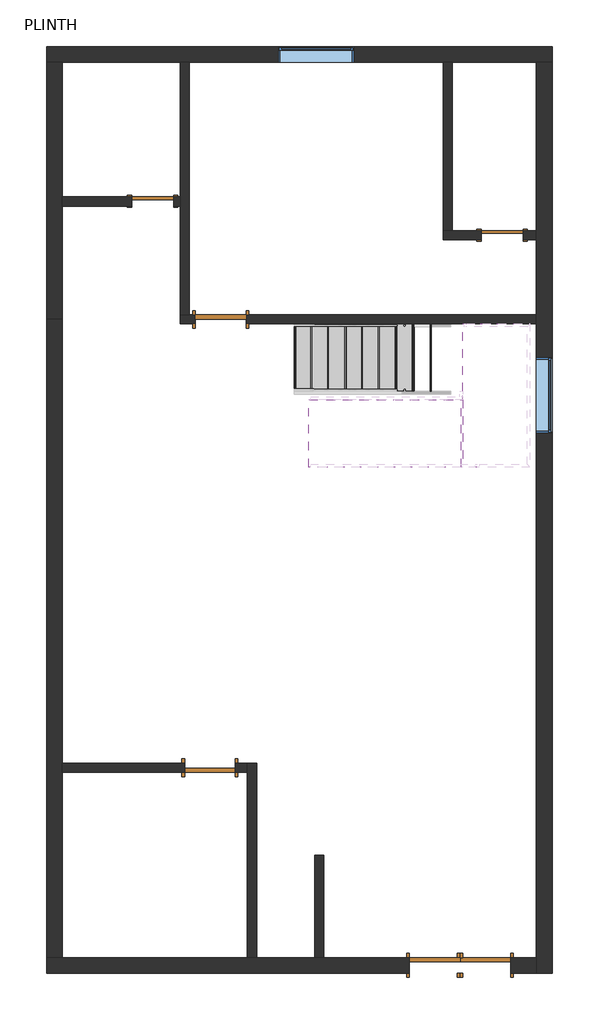
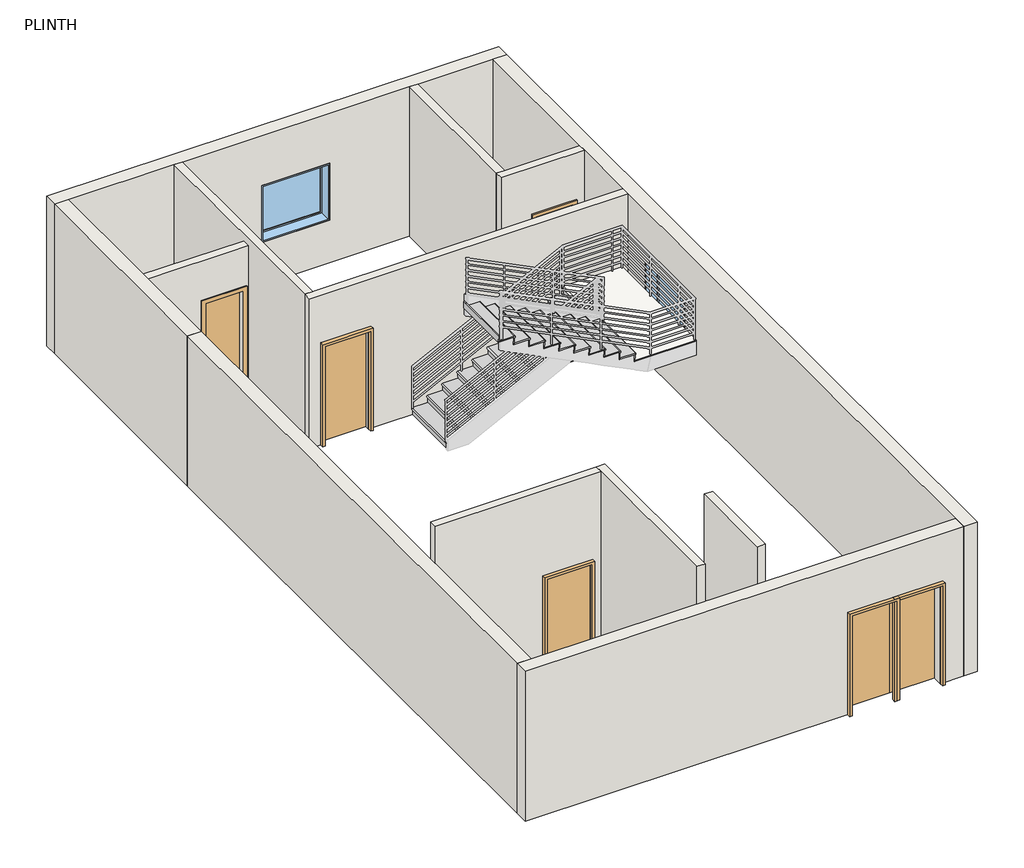
# One storey, part 1 of 4: 13 walls, 6 doors, 2 stair flights, 2 windows, 1 slab.
"""IFC4 building model written with IfcOpenShell, lengths in millimetres."""

from ifc_helpers import new_model, si_unit, frame, origin, origin_with_axes, place, context, project, spatial, polyline, outline, extrude, faceted_brep, transform, mapped, element, save
from components import door_e1312905, m_single_flush_3_86d08d0d, m_single_flush_3_17564fc7, m_single_flush_3_bd8c2fc5, non_monolithic_landing_c74da7f8, stair_flight_50mm_tread_25mm_nosing_13mm_riser_a6b179a3, stair_flight_50mm_tread_25mm_nosing_13mm_riser_e3034239, window_6cb3df29

model = new_model("IFC4")

# Units and contexts
model_context = context("Model", 3, world=origin())
ifc_project = project(units=[si_unit("LENGTHUNIT", "METRE", prefix="MILLI")], contexts=[model_context])

# Site, building, storey
site = spatial("IfcSite", under=ifc_project)
building = spatial("IfcBuilding", under=site)
storey = spatial("IfcBuildingStorey", under=building, Name="PLINTH", Elevation=0.0)

# Doors
placement = place(None, origin())
door_shape = door_e1312905(model_context)
element("IfcDoor", 1, ObjectType="M_Single-Flush : 2'6\"", at=placement, inside=storey, context=model_context, shape_type="MappedRepresentation", body=[
    mapped(door_shape, transform((10612.5583908, 5233.3640673, 0.0), x_axis=(1.0, 0.0, 0.0), y_axis=(0.0, 1.0, 0.0), z_axis=(0.0, 0.0, 1.0))),
])
element("IfcDoor", 2, ObjectType="M_Single-Flush : 2'6\"", at=placement, inside=storey, context=model_context, shape_type="MappedRepresentation", body=[
    mapped(door_shape, transform((4290.0583908, 5842.9640673, 0.0), x_axis=(1.0, 0.0, 0.0), y_axis=(0.0, 1.0, 0.0), z_axis=(0.0, 0.0, 1.0))),
])
m_single_flush_3_shape = m_single_flush_3_86d08d0d(model_context)
element("IfcDoor", 3, ObjectType="M_Single-Flush : 3'", at=placement, inside=storey, context=model_context, shape_type="MappedRepresentation", body=[
    mapped(m_single_flush_3_shape, transform((5522.6583908, 3709.3640673, 0.0), x_axis=(-1.0, 0.0, 0.0), y_axis=(0.0, -1.0, 0.0), z_axis=(0.0, 0.0, 1.0))),
])
element("IfcDoor", 4, ObjectType="M_Single-Flush : 3'", at=placement, inside=storey, context=model_context, shape_type="MappedRepresentation", body=[
    mapped(m_single_flush_3_shape, transform((5325.4583908, -4402.4359327, 0.0), x_axis=(1.0, 0.0, 0.0), y_axis=(0.0, 1.0, 0.0), z_axis=(0.0, 0.0, 1.0))),
])
m_single_flush_3_2_shape = m_single_flush_3_17564fc7(model_context)
element("IfcDoor", 5, ObjectType="M_Single-Flush : 3'", at=placement, inside=storey, context=model_context, shape_type="MappedRepresentation", body=[
    mapped(m_single_flush_3_2_shape, transform((10307.7583908, -7978.5359327, 0.0), x_axis=(1.0, 0.0, 0.0), y_axis=(0.0, 1.0, 0.0), z_axis=(0.0, 0.0, 1.0))),
])
m_single_flush_3_3_shape = m_single_flush_3_bd8c2fc5(model_context)
element("IfcDoor", 6, ObjectType="M_Single-Flush : 3'", at=placement, inside=storey, context=model_context, shape_type="MappedRepresentation", body=[
    mapped(m_single_flush_3_3_shape, transform((9393.3583908, -7978.5359327, 0.0), x_axis=(-1.0, 0.0, 0.0), y_axis=(0.0, -1.0, 0.0), z_axis=(0.0, 0.0, 1.0))),
])

# Slab
non_monolithic_landing_shape = non_monolithic_landing_c74da7f8(model_context)
element("IfcSlab", 7, ObjectType="Non-Monolithic Landing", at=placement, inside=storey, context=model_context, shape_type="MappedRepresentation", body=[
    mapped(non_monolithic_landing_shape, transform((0.0, 0.0, 0.0), x_axis=(1.0, 0.0, 0.0), y_axis=(0.0, 1.0, 0.0), z_axis=(0.0, 0.0, 1.0))),
])

# Stair flights
stair_flight_50mm_tread_25mm_nosing_13mm_riser_shape = stair_flight_50mm_tread_25mm_nosing_13mm_riser_a6b179a3(model_context)
element("IfcStairFlight", 8, ObjectType="50mm Tread 25mm Nosing 13mm Riser", at=placement, inside=storey, context=model_context, shape_type="MappedRepresentation", body=[
    mapped(stair_flight_50mm_tread_25mm_nosing_13mm_riser_shape, transform((0.0, 0.0, 0.0), x_axis=(1.0, 0.0, 0.0), y_axis=(0.0, 1.0, 0.0), z_axis=(0.0, 0.0, 1.0))),
])
stair_flight_50mm_tread_25mm_nosing_13mm_riser_2_shape = stair_flight_50mm_tread_25mm_nosing_13mm_riser_e3034239(model_context)
element("IfcStairFlight", 9, ObjectType="50mm Tread 25mm Nosing 13mm Riser", at=placement, inside=storey, context=model_context, shape_type="MappedRepresentation", body=[
    mapped(stair_flight_50mm_tread_25mm_nosing_13mm_riser_2_shape, transform((0.0, 0.0, 0.0), x_axis=(1.0, 0.0, 0.0), y_axis=(0.0, 1.0, 0.0), z_axis=(0.0, 0.0, 1.0))),
])

# Walls
element("IfcWall", 10, ObjectType="115 MM WALL", at=placement, inside=storey, context=model_context, shape_type="Brep", body=[
    faceted_brep([(4785.3583908, 3626.4640673, 0.0), (5065.4583908, 3626.4640673, 0.0), (5065.4583908, 3626.4640673, 2133.6), (5979.8583908, 3626.4640673, 2133.6), (5979.8583908, 3626.4640673, 0.0), (11234.1583908, 3626.4640673, 0.0), (11234.1583908, 3626.4640673, 3200.4), (4785.3583908, 3626.4640673, 3200.4), (5065.4583908, 3792.2640673, 2133.6), (5065.4583908, 3792.2640673, 0.0), (4951.1583908, 3792.2640673, 0.0), (4785.3583908, 3792.2640673, 0.0), (4785.3583908, 3792.2640673, 3200.4), (4951.1583908, 3792.2640673, 3200.4), (11234.1583908, 3792.2640673, 3200.4), (11234.1583908, 3792.2640673, 0.0), (5979.8583908, 3792.2640673, 0.0), (5979.8583908, 3792.2640673, 2133.6)], [[[0, 1, 2, 3, 4, 5, 6, 7]], [[8, 9, 10, 11, 12, 13, 14, 15, 16, 17]], [[16, 15, 5, 4]], [[11, 10, 9, 1, 0]], [[7, 6, 14, 13, 12]], [[6, 5, 15, 14]], [[0, 7, 12, 11]], [[2, 1, 9, 8]], [[3, 2, 8, 17]], [[4, 3, 17, 16]]]),
])
element("IfcWall", 11, ObjectType="115 MM WALL", at=placement, inside=storey, context=model_context, shape_type="Brep", body=[
    faceted_brep([(4951.1583908, 3792.2640673, 0.0), (4951.1583908, 8364.2640673, 0.0), (4951.1583908, 8364.2640673, 3200.4), (4951.1583908, 3792.2640673, 3200.4), (4785.3583908, 3792.2640673, 0.0), (4785.3583908, 3792.2640673, 3200.4), (4785.3583908, 8364.2640673, 3200.4), (4785.3583908, 8364.2640673, 0.0), (4785.3583908, 5925.8640673, 0.0), (4785.3583908, 5760.0640673, 0.0)], [[[0, 1, 2, 3]], [[4, 5, 6, 7, 8, 9]], [[1, 0, 4, 9, 8, 7]], [[3, 2, 6, 5]], [[2, 1, 7, 6]], [[0, 3, 5, 4]]]),
])
element("IfcWall", 12, ObjectType="115 MM WALL", at=placement, inside=storey, context=model_context, shape_type="SweptSolid", body=[
    extrude(outline(polyline([(9544.3583908, 5316.2640673), (9544.3583908, 8364.2640673), (9710.1583908, 8364.2640673), (9710.1583908, 5316.2640673), (9544.3583908, 5316.2640673)])), origin_with_axes(), (0.0, 0.0, 1.0), 3200.4),
])
element("IfcWall", 13, ObjectType="115 MM WALL", at=placement, inside=storey, context=model_context, shape_type="Brep", body=[
    faceted_brep([(10993.5583908, 5150.4640673, 2133.6), (10993.5583908, 5150.4640673, 0.0), (11234.1583908, 5150.4640673, 0.0), (11234.1583908, 5150.4640673, 3200.4), (9544.3583908, 5150.4640673, 3200.4), (9544.3583908, 5150.4640673, 0.0), (10231.5583908, 5150.4640673, 0.0), (10231.5583908, 5150.4640673, 2133.6), (11234.1583908, 5316.2640673, 0.0), (10993.5583908, 5316.2640673, 0.0), (10993.5583908, 5316.2640673, 2133.6), (10231.5583908, 5316.2640673, 2133.6), (10231.5583908, 5316.2640673, 0.0), (9710.1583908, 5316.2640673, 0.0), (9544.3583908, 5316.2640673, 0.0), (9544.3583908, 5316.2640673, 3200.4), (9710.1583908, 5316.2640673, 3200.4), (11234.1583908, 5316.2640673, 3200.4)], [[[0, 1, 2, 3, 4, 5, 6, 7]], [[8, 9, 10, 11, 12, 13, 14, 15, 16, 17]], [[6, 5, 14, 13, 12]], [[2, 1, 9, 8]], [[4, 3, 17, 16, 15]], [[3, 2, 8, 17]], [[5, 4, 15, 14]], [[10, 9, 1, 0]], [[11, 10, 0, 7]], [[12, 11, 7, 6]]]),
])
element("IfcWall", 14, ObjectType="115 MM WALL", at=placement, inside=storey, context=model_context, shape_type="SweptSolid", body=[
    extrude(outline(polyline([(2133.6, 4671.0583908), (0.0, 4671.0583908), (0.0, 4785.3583908), (3048.0, 4785.3583908), (3048.0, 2651.7583908), (0.0, 2651.7583908), (0.0, 3909.0583908), (2133.6, 3909.0583908), (2133.6, 4671.0583908)])), frame((0.0, 5760.0640673, 0.0), z_axis=(0.0, 1.0, 0.0), x_axis=(0.0, 0.0, 1.0)), (0.0, 0.0, 1.0), 165.8),
])
element("IfcWall", 15, ObjectType="115 MM WALL", at=placement, inside=storey, context=model_context, shape_type="Brep", body=[
    faceted_brep([(6170.3583908, -7838.1359327, 0.0), (6170.3583908, -4319.5359327, 0.0), (6170.3583908, -4319.5359327, 4000.0), (6170.3583908, -7838.1359327, 4000.0), (6004.5583908, -7838.1359327, 0.0), (6004.5583908, -7838.1359327, 4000.0), (6004.5583908, -4485.3359327, 4000.0), (6004.5583908, -4319.5359327, 4000.0), (6004.5583908, -4319.5359327, 0.0), (6004.5583908, -4485.3359327, 0.0)], [[[0, 1, 2, 3]], [[4, 5, 6, 7, 8, 9]], [[1, 0, 4, 9, 8]], [[3, 2, 7, 6, 5]], [[0, 3, 5, 4]], [[2, 1, 8, 7]]]),
])
element("IfcWall", 16, ObjectType="115 MM WALL", at=placement, inside=storey, context=model_context, shape_type="SweptSolid", body=[
    extrude(outline(polyline([(2133.6, 5782.6583908), (0.0, 5782.6583908), (0.0, 6004.5583908), (4000.0, 6004.5583908), (4000.0, 2651.7583908), (0.0, 2651.7583908), (0.0, 4868.2583908), (2133.6, 4868.2583908), (2133.6, 5782.6583908)])), frame((0.0, -4485.3359327, 0.0), z_axis=(0.0, 1.0, 0.0), x_axis=(0.0, 0.0, 1.0)), (0.0, 0.0, 1.0), 165.8),
])
element("IfcWall", 17, ObjectType="115 MM WALL", at=placement, inside=storey, context=model_context, shape_type="SweptSolid", body=[
    extrude(outline(polyline([(7389.5583908, -5985.3359327), (7389.5583908, -7838.1359327), (7223.7583908, -7838.1359327), (7223.7583908, -5985.3359327), (7389.5583908, -5985.3359327)])), origin_with_axes(), (0.0, 0.0, 1.0), 4000.0),
])
element("IfcWall", 18, ObjectType="230MM WALL", at=placement, inside=storey, context=model_context, shape_type="Brep", body=[
    faceted_brep([(2370.9583908, 8364.2640673, 0.0), (2651.7583908, 8364.2640673, 0.0), (4785.3583908, 8364.2640673, 0.0), (4951.1583908, 8364.2640673, 0.0), (9544.3583908, 8364.2640673, 0.0), (9710.1583908, 8364.2640673, 0.0), (11234.1583908, 8364.2640673, 0.0), (11514.9583908, 8364.2640673, 0.0), (11514.9583908, 8364.2640673, 3200.4), (11234.1583908, 8364.2640673, 3200.4), (9710.1583908, 8364.2640673, 3200.4), (9544.3583908, 8364.2640673, 3200.4), (4951.1583908, 8364.2640673, 3200.4), (4785.3583908, 8364.2640673, 3200.4), (2651.7583908, 8364.2640673, 3200.4), (2370.9583908, 8364.2640673, 3200.4), (6561.9583908, 8364.2640673, 914.4), (6561.9583908, 8364.2640673, 2133.6), (7933.5583908, 8364.2640673, 2133.6), (7933.5583908, 8364.2640673, 914.4), (2370.9583908, 8645.0640673, 0.0), (2370.9583908, 8645.0640673, 3200.4), (11514.9583908, 8645.0640673, 3200.4), (11514.9583908, 8645.0640673, 0.0), (6561.9583908, 8645.0640673, 914.4), (7933.5583908, 8645.0640673, 914.4), (7933.5583908, 8645.0640673, 2133.6), (6561.9583908, 8645.0640673, 2133.6)], [[[0, 1, 2, 3, 4, 5, 6, 7, 8, 9, 10, 11, 12, 13, 14, 15], [16, 17, 18, 19]], [[20, 21, 22, 23], [24, 25, 26, 27]], [[7, 6, 5, 4, 3, 2, 1, 0, 20, 23]], [[15, 14, 13, 12, 11, 10, 9, 8, 22, 21]], [[8, 7, 23, 22]], [[0, 15, 21, 20]], [[17, 16, 24, 27]], [[18, 17, 27, 26]], [[19, 18, 26, 25]], [[16, 19, 25, 24]]]),
])
element("IfcWall", 19, ObjectType="230MM WALL", at=placement, inside=storey, context=model_context, shape_type="Brep", body=[
    faceted_brep([(11234.1583908, 8364.2640673, 0.0), (11234.1583908, 5316.2640673, 0.0), (11234.1583908, 5150.4640673, 0.0), (11234.1583908, 3792.2640673, 0.0), (11234.1583908, 3626.4640673, 0.0), (11234.1583908, -7838.1359327, 0.0), (11234.1583908, -8118.9359327, 0.0), (11234.1583908, -8118.9359327, 3200.4), (11234.1583908, -7838.1359327, 3200.4), (11234.1583908, 3626.4640673, 3200.4), (11234.1583908, 3792.2640673, 3200.4), (11234.1583908, 5150.4640673, 3200.4), (11234.1583908, 5316.2640673, 3200.4), (11234.1583908, 8364.2640673, 3200.4), (11234.1583908, 3023.5640673, 914.4), (11234.1583908, 3023.5640673, 2133.6), (11234.1583908, 1651.9640673, 2133.6), (11234.1583908, 1651.9640673, 914.4), (11514.9583908, 8364.2640673, 0.0), (11514.9583908, 8364.2640673, 3200.4), (11514.9583908, -8118.9359327, 3200.4), (11514.9583908, -8118.9359327, 0.0), (11514.9583908, 3023.5640673, 914.4), (11514.9583908, 1651.9640673, 914.4), (11514.9583908, 1651.9640673, 2133.6), (11514.9583908, 3023.5640673, 2133.6)], [[[0, 1, 2, 3, 4, 5, 6, 7, 8, 9, 10, 11, 12, 13], [14, 15, 16, 17]], [[18, 19, 20, 21], [22, 23, 24, 25]], [[6, 5, 4, 3, 2, 1, 0, 18, 21]], [[13, 12, 11, 10, 9, 8, 7, 20, 19]], [[0, 13, 19, 18]], [[7, 6, 21, 20]], [[15, 14, 22, 25]], [[16, 15, 25, 24]], [[17, 16, 24, 23]], [[14, 17, 23, 22]]]),
])
element("IfcWall", 20, ObjectType="230MM WALL", at=placement, inside=storey, context=model_context, shape_type="Brep", body=[
    faceted_brep([(2370.9583908, -7838.1359327, 3200.4), (2651.7583908, -7838.1359327, 3200.4), (11234.1583908, -7838.1359327, 3200.4), (11234.1583908, -7838.1359327, 0.0), (10764.9583908, -7838.1359327, 0.0), (10764.9583908, -7838.1359327, 2133.6), (8936.1583908, -7838.1359327, 2133.6), (8936.1583908, -7838.1359327, 0.0), (7389.5583908, -7838.1359327, 0.0), (7223.7583908, -7838.1359327, 0.0), (6170.3583908, -7838.1359327, 0.0), (6004.5583908, -7838.1359327, 0.0), (2651.7583908, -7838.1359327, 0.0), (2370.9583908, -7838.1359327, 0.0), (11234.1583908, -8118.9359327, 3200.4), (2370.9583908, -8118.9359327, 3200.4), (2370.9583908, -8118.9359327, 0.0), (8936.1583908, -8118.9359327, 0.0), (8936.1583908, -8118.9359327, 2133.6), (10764.9583908, -8118.9359327, 2133.6), (10764.9583908, -8118.9359327, 0.0), (11234.1583908, -8118.9359327, 0.0)], [[[0, 1, 2, 3, 4, 5, 6, 7, 8, 9, 10, 11, 12, 13]], [[14, 15, 16, 17, 18, 19, 20, 21]], [[3, 21, 20, 4]], [[16, 13, 12, 11, 10, 9, 8, 7, 17]], [[2, 1, 0, 15, 14]], [[3, 2, 14, 21]], [[0, 13, 16, 15]], [[5, 4, 20, 19]], [[5, 19, 18, 6]], [[6, 18, 17, 7]]]),
])
element("IfcWall", 21, ObjectType="230MM WALL", at=placement, inside=storey, context=model_context, shape_type="Brep", body=[
    faceted_brep([(2651.7583908, -7838.1359327, 0.0), (2651.7583908, -4485.3359327, 0.0), (2651.7583908, -4319.5359327, 0.0), (2651.7583908, 3709.3640673, 0.0), (2651.7583908, 3709.3640673, 3200.4), (2651.7583908, -7838.1359327, 3200.4), (2370.9583908, -7838.1359327, 0.0), (2370.9583908, -7838.1359327, 3200.4), (2370.9583908, 3709.3640673, 3200.4), (2370.9583908, 3709.3640673, 0.0)], [[[0, 1, 2, 3, 4, 5]], [[6, 7, 8, 9]], [[3, 2, 1, 0, 6, 9]], [[4, 3, 9, 8]], [[5, 4, 8, 7]], [[0, 5, 7, 6]]]),
])
element("IfcWall", 22, ObjectType="230MM WALL", at=placement, inside=storey, context=model_context, shape_type="Brep", body=[
    faceted_brep([(2651.7583908, 3709.3640673, 0.0), (2651.7583908, 5760.0640673, 0.0), (2651.7583908, 5925.8640673, 0.0), (2651.7583908, 8364.2640673, 0.0), (2651.7583908, 8364.2640673, 3200.4), (2651.7583908, 3709.3640673, 3200.4), (2370.9583908, 3709.3640673, 0.0), (2370.9583908, 3709.3640673, 3200.4), (2370.9583908, 8364.2640673, 3200.4), (2370.9583908, 8364.2640673, 0.0)], [[[0, 1, 2, 3, 4, 5]], [[6, 7, 8, 9]], [[3, 2, 1, 0, 6, 9]], [[5, 4, 8, 7]], [[0, 5, 7, 6]], [[4, 3, 9, 8]]]),
])

# Windows
window_shape = window_6cb3df29(model_context)
element("IfcWindow", 23, ObjectType="M_Fixed : 4'6\"X4'", at=placement, inside=storey, context=model_context, shape_type="MappedRepresentation", body=[
    mapped(window_shape, transform((7247.7583908, 8491.6640673, 0.0), x_axis=(1.0, 0.0, 0.0), y_axis=(0.0, 1.0, 0.0), z_axis=(0.0, 0.0, 1.0))),
])
element("IfcWindow", 24, ObjectType="M_Fixed : 4'6\"X4'", at=placement, inside=storey, context=model_context, shape_type="MappedRepresentation", body=[
    mapped(window_shape, transform((11361.5583908, 2337.7640673, 0.0), x_axis=(0.0, -1.0, 0.0), y_axis=(1.0, 0.0, 0.0), z_axis=(0.0, 0.0, 1.0))),
])

save(model, "model.ifc")

# Revit data of these elements
# Type "M_Single-Flush : 2'6\""
#   Type Mark = "22"
#   Thickness = 0' - 2.00787"
#   Height = 7' - 0"
#   Trim Projection Ext = 0' - 0.98425"
#   Trim Projection Int = 0' - 0.98425"
#   Trim Width = 0' - 2.99213"
#   Width = 2' - 6"
#   Door Material = Door - Panel
#   Frame Material = Door - Frame
#   Function = (empty or 0)
#   Wall Closure = (empty or 0)
# Type "M_Single-Flush : 3'"
#   Type Mark = "23"
#   Thickness = 0' - 3"
#   Height = 7' - 0"
#   Trim Projection Ext = 0' - 3"
#   Trim Projection Int = 0' - 3"
#   Trim Width = 0' - 2"
#   Width = 3' - 0"
#   Wall Closure = 2
#   Door Material = Door - Panel
#   Frame Material = Door - Panel
#   Function = (empty or 0)
# Type "115 MM WALL"
#   Layers, outside or top first: 0' - 1" "PLASTER OUTSIDE" (function 4); 0' - 4 135/256" "Brick, Common" (function 1); 0' - 1" "PLASTER INSIDE" (function 5)
# Type "230MM WALL"
#   Layers, outside or top first: 0' - 1" "PLASTER OUTSIDE" (function 4); 0' - 9 7/128" "Brick, Common" (function 1); 0' - 1" "PLASTER INSIDE" (function 5)
# Type "M_Fixed : 4'6\"X4'"
#   Construction Type Id = "DG-DR"
#   Analytic Construction = "Double glazing - domestic"
#   Type Mark = "19"
#   Visual Light Transmittance = 0.81
#   Solar Heat Gain Coefficient = 0.76
#   Heat Transfer Coefficient (U) = 3.1292 W/(m²·K)
#   Height = 4' - 0"
#   Default Sill Height = 3' - 0"
#   Width = 4' - 6"
#   Window Inset = 0' - 0.74803"
#   Wall Closure = 2
#   Frame Exterior Material = Sash
#   Frame Interior Material = Sash
#   Glass Pane Material = Glass
#   Sash = Sash
# Elements 1, 2 (IfcDoor, "M_Single-Flush : 2'6\"")
#   Phase Created = New Construction
#   Materials on its faces: "Door - Frame", "Door - Panel"
# Elements 3, 4, 5, 6 (IfcDoor, "M_Single-Flush : 3'")
#   Phase Created = New Construction
#   Materials on its faces: "Door - Panel"
# Element 7 (IfcSlab, "Non-Monolithic Landing")
#   Phase Created = New Construction
# Elements 8, 9 (IfcStairFlight, "50mm Tread 25mm Nosing 13mm Riser")
#   Phase Created = New Construction
# Elements 10, 11, 12, 13 (IfcWall, "115 MM WALL")
#   Top Offset = 0' - 0"
#   Base Offset = 0' - 0"
#   Unconnected Height = 10' - 6"
#   wall height = 10' - 6"
#   Phase Created = New Construction
#   Base Constraint = PLINTH
#   Materials on its faces: "PLASTER INSIDE", "PLASTER OUTSIDE"
# Element 14 (IfcWall, "115 MM WALL")
#   Top Offset = 0' - 0"
#   Base Offset = 0' - 0"
#   Unconnected Height = 10' - 0"
#   wall height = 10' - 0"
#   Phase Created = New Construction
#   Base Constraint = PLINTH
#   Materials on its faces: "PLASTER INSIDE", "PLASTER OUTSIDE"
# Elements 15, 16, 17 (IfcWall, "115 MM WALL")
#   Top Offset = 0' - 0"
#   Base Offset = 0' - 0"
#   Unconnected Height = 13' - 1.48031"
#   wall height = 13' - 1.48031"
#   Phase Created = New Construction
#   Base Constraint = PLINTH
#   Materials on its faces: "PLASTER INSIDE", "PLASTER OUTSIDE"
# Elements 18, 19, 20 (IfcWall, "230MM WALL")
#   Top Offset = 0' - 0"
#   Base Offset = 0' - 0"
#   Unconnected Height = 10' - 6"
#   wall height = 10' - 6"
#   Phase Created = New Construction
#   Base Constraint = PLINTH
#   Materials on its faces: "Default Wall", "PLASTER OUTSIDE", "PLASTER INSIDE"
# Elements 21, 22 (IfcWall, "230MM WALL")
#   Top Offset = 0' - 0"
#   Base Offset = 0' - 0"
#   Unconnected Height = 10' - 6"
#   wall height = 10' - 6"
#   Phase Created = New Construction
#   Base Constraint = PLINTH
#   Materials on its faces: "Default Wall", "PLASTER INSIDE", "PLASTER OUTSIDE"
# Element 23 (IfcWindow, "M_Fixed : 4'6\"X4'")
#   Mark = "6"
#   Phase Created = New Construction
#   Materials on its faces: "Sash", "Glass"
# Element 24 (IfcWindow, "M_Fixed : 4'6\"X4'")
#   Mark = "7"
#   Phase Created = New Construction
#   Materials on its faces: "Sash", "Glass"
# Materials
#   "Door - Panel": class "Wood", colour RGB 114 82 51, transparency 0
#   "Door - Frame": colour RGB 153 76 43, transparency 0
#   "PLASTER OUTSIDE": class "Concrete", colour RGB 215 204 180, transparency 0, Cost = 0
#   "Brick, Common": class "Masonry", colour RGB 76 55 59, transparency 0, Description = "Common brick", Cost = 0
#   "PLASTER INSIDE": class "Generic", colour RGB 215 204 180, transparency 0, Cost = 0
#   "Sash": class "Wood", colour RGB 136 99 55, transparency 0
#   "Glass": class "Glass", colour RGB 218 227 224, transparency 0.85, Description = "Soda Lime Glass", Cost = 0
#   "Default Wall": colour RGB 80 80 80, transparency 0
